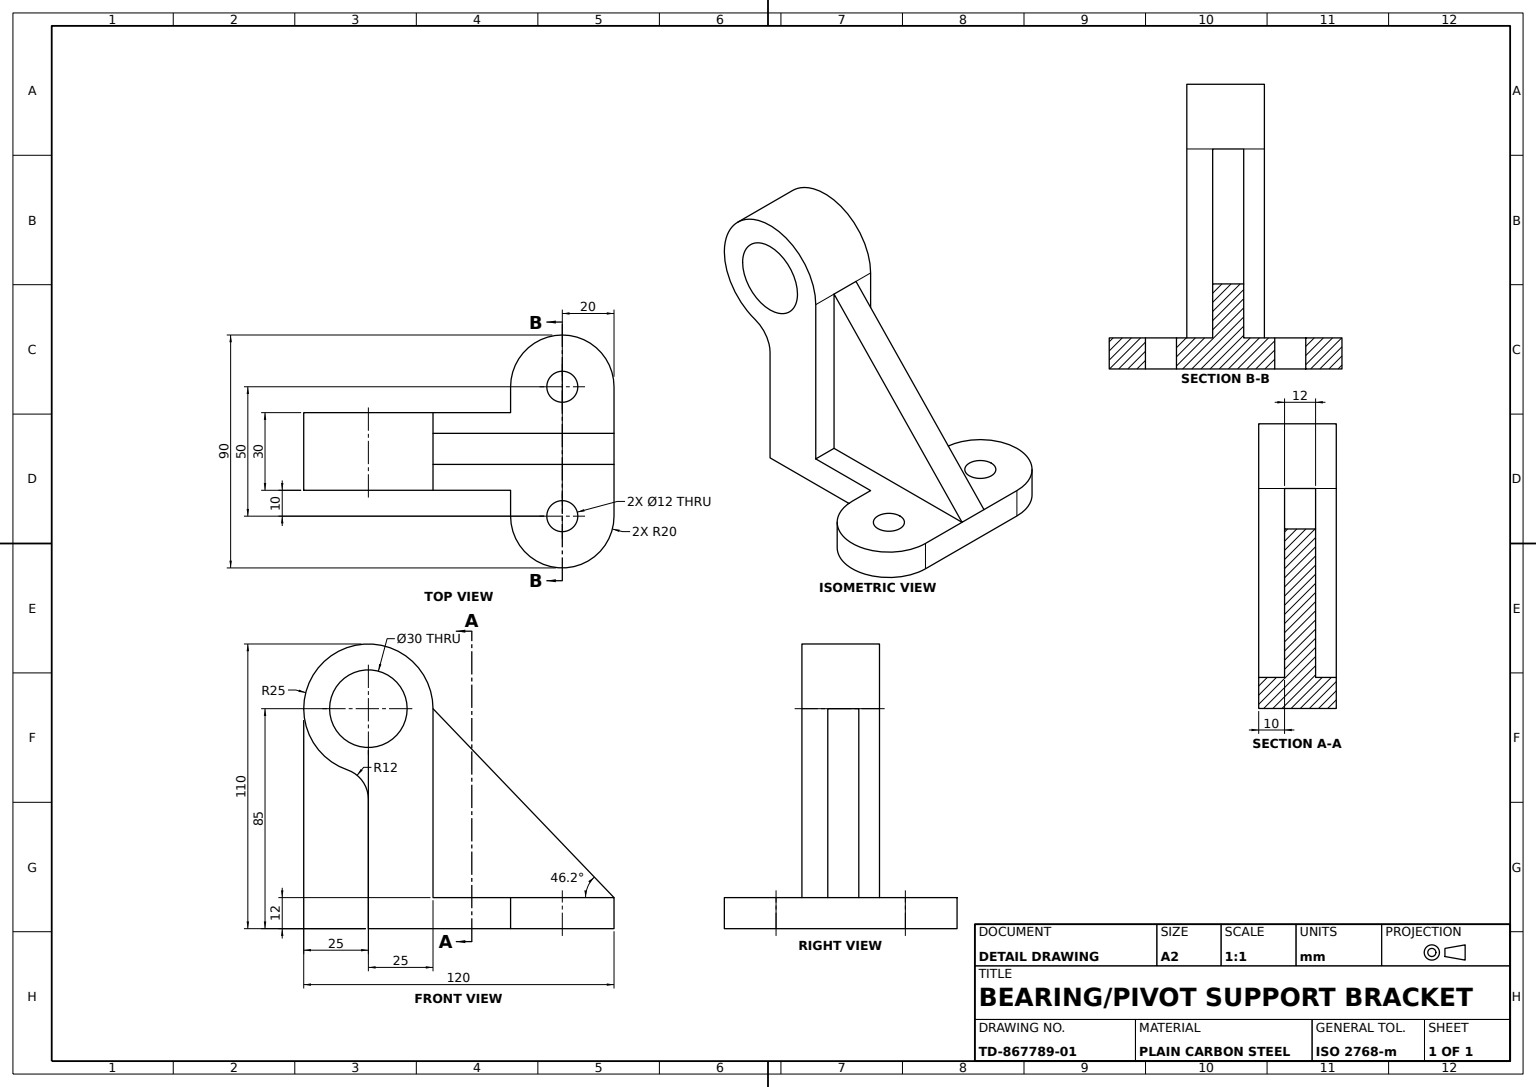
from build123d import *

# Parameters (mm, degrees)
BASE_PLATE_SKETCH_R     = 6
BASE_PLATE_DEPTH        = 6
UPRIGHT_BORE_SKETCH_R   = 15
UPRIGHT_WITH_BORE_DEPTH = 15
RIB_SKETCH_W            = 12
RIB_SKETCH_H            = 73
RIB_DEPTH               = 70
RIB_WEDGE_CUT_DEPTH     = 70


with BuildPart() as part:
    # Base Plate Sketch → Base Plate (new, symmetric)
    with BuildSketch(Plane(origin=(0, 0, 0), x_dir=(1, 0, 0), z_dir=(0, 1, 0))):
        with BuildLine():
            Line((-20, 25), (-20, 15))
            Line((-20, 15), (-50, 15))
            Line((-50, 15), (-50, -15))
            Line((-50, -15), (-20, -15))
            Line((-20, -15), (-20, -25))
            ThreePointArc((-20, -25), (0, -45), (20, -25))
            Line((20, -25), (20, 25))
            ThreePointArc((20, 25), (0, 45), (-20, 25))
        make_face()
        with Locations(Location((0, 25, 0), (0, 0, 270))):
            Circle(BASE_PLATE_SKETCH_R, mode=Mode.SUBTRACT)
        with Locations(Location((0, -25, 0), (0, 0, 270))):
            Circle(BASE_PLATE_SKETCH_R, mode=Mode.SUBTRACT)
    extrude(amount=BASE_PLATE_DEPTH, both=True)

    # Upright Bore Sketch → Upright with Bore (add, symmetric)
    with BuildSketch(Plane.XY):
        with BuildLine():
            Line((-50, -6), (-75, -6))
            Line((-75, -6), (-75, 44))
            ThreePointArc((-75, 44), (-77.235198346, 50.974858325), (-83.108108108, 55.351351351))
            ThreePointArc((-83.108108108, 55.351351351), (-89.530954843, 99.34333678), (-50, 79))
            Line((-50, 79), (-50, -6))
        make_face()
        with Locations((-75, 79)):
            Circle(UPRIGHT_BORE_SKETCH_R, mode=Mode.SUBTRACT)
    extrude(amount=UPRIGHT_WITH_BORE_DEPTH, both=True)

    # Rib Sketch → Rib (add)
    with BuildSketch(Plane(origin=(-50, 0, 0), x_dir=(0, 0, -1), z_dir=(1, 0, 0))):
        with Locations((1, 42.5)):
            Rectangle(RIB_SKETCH_W, RIB_SKETCH_H)
    extrude(amount=RIB_DEPTH)

    # Rib Wedge Cut Sketch → Rib Wedge Cut (cut)
    with BuildSketch(Plane.XY.offset(5)):
        Polygon((20, 6), (-50, 79), (20, 79), align=None)
    extrude(amount=-RIB_WEDGE_CUT_DEPTH, mode=Mode.SUBTRACT)


solid = part.part
